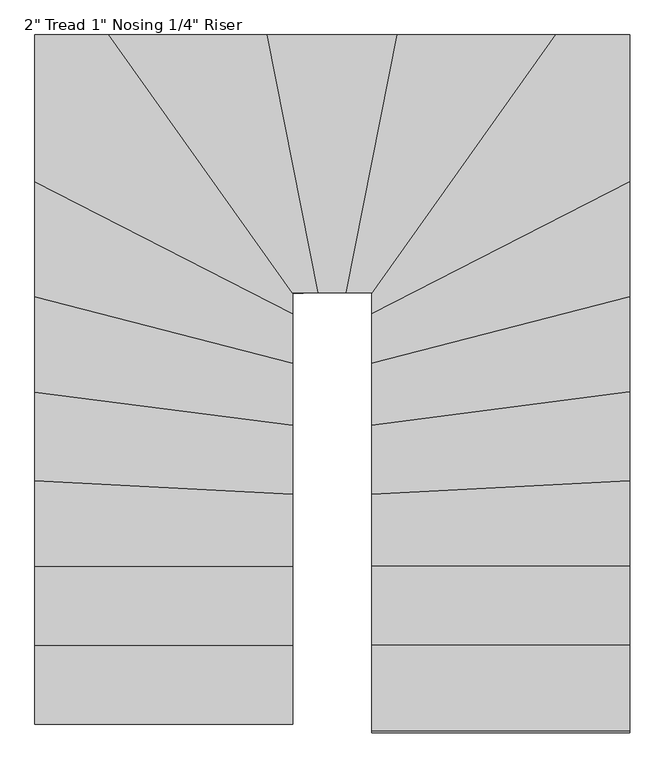
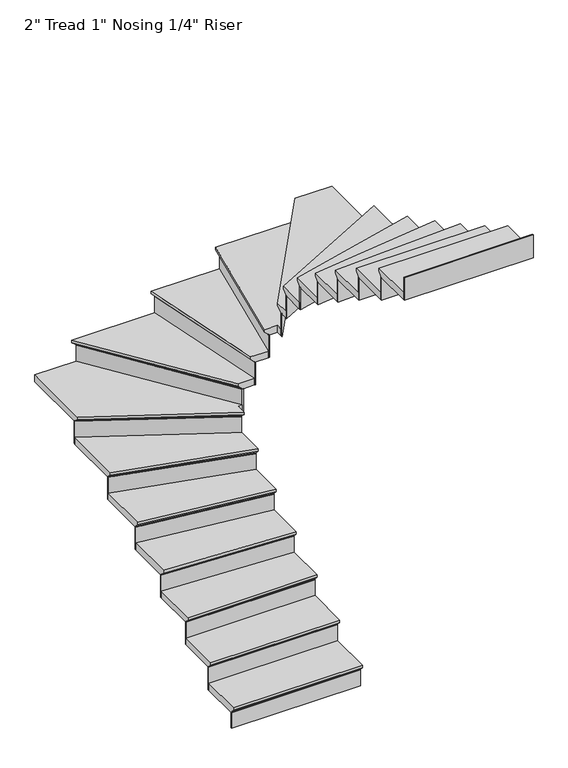
"""IFC4 building model written with IfcOpenShell, lengths in millimetres: stair flight geometry."""

from ifc_helpers import new_model, si_unit, origin, place, context, project, spatial, faceted_brep, source, transform, mapped, element, save


def stair_flight_4b86e887(model_context):
    return source(origin(), model_context, "Body", "Brep", [
        faceted_brep([(-715.0890964, 3647.9718401, 3350.6833333), (-715.0890964, 3647.9718401, 3369.7333333), (-1629.4890964, 3647.9718401, 3369.7333333), (-1629.4890964, 3647.9718401, 3350.6833333), (-715.0890964, 3673.3718401, 3325.2833333), (-1629.4890964, 3673.3718401, 3325.2833333), (-715.0890964, 3952.7718401, 3369.7333333), (-1629.4890964, 3952.7718401, 3369.7333333), (-1629.4890964, 3673.3718401, 3318.9333333), (-1629.4890964, 3952.7718401, 3318.9333333), (-715.0890964, 3952.7718401, 3318.9333333), (-715.0890964, 3673.3718401, 3318.9333333)], [[[0, 1, 2, 3]], [[4, 0, 3, 5]], [[2, 1, 6, 7]], [[8, 9, 10, 11]], [[2, 7, 9, 8, 5, 3]], [[8, 11, 4, 5]], [[6, 1, 0, 4, 11, 10]], [[7, 6, 10, 9]]]),
        faceted_brep([(-715.0890964, 3673.3718401, 3318.9333333), (-715.0890964, 3673.3718401, 3200.4), (-715.0890964, 3679.7218401, 3200.4), (-715.0890964, 3679.7218401, 3318.9333333), (-1629.4890964, 3673.3718401, 3318.9333333), (-1629.4890964, 3679.7218401, 3318.9333333), (-1629.4890964, 3679.7218401, 3200.4), (-1629.4890964, 3673.3718401, 3200.4)], [[[0, 1, 2, 3]], [[4, 5, 6, 7]], [[1, 0, 4, 7]], [[2, 1, 7, 6]], [[3, 2, 6, 5]], [[0, 3, 5, 4]]]),
        faceted_brep([(-715.0890964, 3952.7718401, 3488.2666667), (-715.0890964, 3952.7718401, 3318.9333333), (-715.0890964, 3959.1218401, 3318.9333333), (-715.0890964, 3959.1218401, 3488.2666667), (-1629.4890964, 3952.7718401, 3488.2666667), (-1629.4890964, 3959.1218401, 3488.2666667), (-1629.4890964, 3959.1218401, 3318.9333333), (-1629.4890964, 3952.7718401, 3318.9333333)], [[[0, 1, 2, 3]], [[4, 5, 6, 7]], [[1, 0, 4, 7]], [[2, 1, 7, 6]], [[3, 2, 6, 5]], [[0, 3, 5, 4]]]),
        faceted_brep([(-1629.4890964, 3927.3718401, 3539.0666667), (-715.0890964, 3927.3718401, 3539.0666667), (-715.0890964, 4232.1718401, 3539.0666667), (-1629.4890964, 4232.1718401, 3539.0666667), (-1629.4890964, 3952.7718401, 3488.2666667), (-1629.4890964, 4232.1718401, 3488.2666667), (-715.0890964, 4232.1718401, 3488.2666667), (-715.0890964, 3952.7718401, 3488.2666667), (-1629.4890964, 3952.7718401, 3494.6166667), (-1629.4890964, 3927.3718401, 3520.0166667), (-715.0890964, 3952.7718401, 3494.6166667), (-715.0890964, 3927.3718401, 3520.0166667)], [[[0, 1, 2, 3]], [[4, 5, 6, 7]], [[0, 3, 5, 4, 8, 9]], [[4, 7, 10, 8]], [[2, 1, 11, 10, 7, 6]], [[3, 2, 6, 5]], [[11, 1, 0, 9]], [[10, 11, 9, 8]]]),
        faceted_brep([(-715.0890964, 4232.1718401, 3657.6), (-715.0890964, 4232.1718401, 3488.2666667), (-715.0890964, 4238.5218401, 3488.2666667), (-715.0890964, 4238.5218401, 3657.6), (-1629.4890964, 4232.1718401, 3657.6), (-1629.4890964, 4238.5218401, 3657.6), (-1629.4890964, 4238.5218401, 3488.2666667), (-1629.4890964, 4232.1718401, 3488.2666667)], [[[0, 1, 2, 3]], [[4, 5, 6, 7]], [[1, 0, 4, 7]], [[2, 1, 7, 6]], [[3, 2, 6, 5]], [[0, 3, 5, 4]]]),
        faceted_brep([(-1629.4890964, 4206.7718401, 3708.4), (-715.0890964, 4206.7718401, 3708.4), (-715.0890964, 4487.8390016, 3708.4), (-1629.4890964, 4535.373272, 3708.4), (-1629.4890964, 4232.1718401, 3657.6), (-1629.4890964, 4535.373272, 3657.6), (-715.0890964, 4487.8390016, 3657.6), (-715.0890964, 4232.1718401, 3657.6), (-1629.4890964, 4232.1718401, 3663.95), (-1629.4890964, 4206.7718401, 3689.35), (-715.0890964, 4232.1718401, 3663.95), (-715.0890964, 4206.7718401, 3689.35)], [[[0, 1, 2, 3]], [[4, 5, 6, 7]], [[0, 3, 5, 4, 8, 9]], [[4, 7, 10, 8]], [[2, 1, 11, 10, 7, 6]], [[3, 2, 6, 5]], [[11, 1, 0, 9]], [[10, 11, 9, 8]]]),
        faceted_brep([(-715.0890964, 4487.8390016, 3826.9333333), (-715.0890964, 4487.8390016, 3657.6), (-715.0890964, 4494.1975757, 3657.6), (-715.0890964, 4494.1975757, 3826.9333333), (-1629.4890964, 4535.373272, 3826.9333333), (-1629.4890964, 4541.7318461, 3826.9333333), (-1629.4890964, 4541.7318461, 3657.6), (-1629.4890964, 4535.373272, 3657.6)], [[[0, 1, 2, 3]], [[4, 5, 6, 7]], [[1, 0, 4, 7]], [[2, 1, 7, 6]], [[3, 2, 6, 5]], [[0, 3, 5, 4]]]),
        faceted_brep([(-1629.4890964, 4509.9389753, 3877.7333333), (-715.0890964, 4462.4047049, 3877.7333333), (-715.0890964, 4732.0057014, 3877.7333333), (-1629.4890964, 4850.361753, 3877.7333333), (-1629.4890964, 4535.373272, 3826.9333333), (-1629.4890964, 4850.361753, 3826.9333333), (-715.0890964, 4732.0057014, 3826.9333333), (-715.0890964, 4487.8390016, 3826.9333333), (-1629.4890964, 4535.373272, 3833.2833333), (-1629.4890964, 4509.9389753, 3858.6833333), (-715.0890964, 4487.8390016, 3833.2833333), (-715.0890964, 4462.4047049, 3858.6833333)], [[[0, 1, 2, 3]], [[4, 5, 6, 7]], [[0, 3, 5, 4, 8, 9]], [[4, 7, 10, 8]], [[2, 1, 11, 10, 7, 6]], [[3, 2, 6, 5]], [[11, 1, 0, 9]], [[10, 11, 9, 8]]]),
        faceted_brep([(-715.0890964, 4732.0057014, 3996.2666667), (-715.0890964, 4732.0057014, 3826.9333333), (-715.0890964, 4738.4086732, 3826.9333333), (-715.0890964, 4738.4086732, 3996.2666667), (-1629.4890964, 4850.361753, 3996.2666667), (-1629.4890964, 4856.7647248, 3996.2666667), (-1629.4890964, 4856.7647248, 3826.9333333), (-1629.4890964, 4850.361753, 3826.9333333)], [[[0, 1, 2, 3]], [[4, 5, 6, 7]], [[1, 0, 4, 7]], [[2, 1, 7, 6]], [[3, 2, 6, 5]], [[0, 3, 5, 4]]]),
        faceted_brep([(-1629.4890964, 4824.7498659, 4047.0666667), (-715.0890964, 4706.3938143, 4047.0666667), (-715.0890964, 4953.6329239, 4047.0666667), (-1629.4890964, 5188.7633713, 4047.0666667), (-1629.4890964, 4850.361753, 3996.2666667), (-1629.4890964, 5188.7633713, 3996.2666667), (-715.0890964, 4953.6329239, 3996.2666667), (-715.0890964, 4732.0057014, 3996.2666667), (-1629.4890964, 4850.361753, 4002.6166667), (-1629.4890964, 4824.7498659, 4028.0166667), (-715.0890964, 4732.0057014, 4002.6166667), (-715.0890964, 4706.3938143, 4028.0166667)], [[[0, 1, 2, 3]], [[4, 5, 6, 7]], [[0, 3, 5, 4, 8, 9]], [[4, 7, 10, 8]], [[2, 1, 11, 10, 7, 6]], [[3, 2, 6, 5]], [[11, 1, 0, 9]], [[10, 11, 9, 8]]]),
        faceted_brep([(-715.0890964, 4953.6329239, 4165.6), (-715.0890964, 4953.6329239, 3996.2666667), (-715.0890964, 4960.1895007, 3996.2666667), (-715.0890964, 4960.1895007, 4165.6), (-1629.4890964, 5188.7633713, 4165.6), (-1629.4890964, 5195.3199481, 4165.6), (-1629.4890964, 5195.3199481, 3996.2666667), (-1629.4890964, 5188.7633713, 3996.2666667)], [[[0, 1, 2, 3]], [[4, 5, 6, 7]], [[1, 0, 4, 7]], [[2, 1, 7, 6]], [[3, 2, 6, 5]], [[0, 3, 5, 4]]]),
        faceted_brep([(-1629.4890964, 5162.5370638, 4216.4), (-715.0890964, 4927.4066164, 4216.4), (-715.0890964, 5129.9795599, 4216.4), (-1629.4890964, 5598.8041813, 4216.4), (-1629.4890964, 5188.7633713, 4165.6), (-1629.4890964, 5598.8041813, 4165.6), (-715.0890964, 5129.9795599, 4165.6), (-715.0890964, 4953.6329239, 4165.6), (-1629.4890964, 5188.7633713, 4171.95), (-1629.4890964, 5162.5370638, 4197.35), (-715.0890964, 4953.6329239, 4171.95), (-715.0890964, 4927.4066164, 4197.35)], [[[0, 1, 2, 3]], [[4, 5, 6, 7]], [[0, 3, 5, 4, 8, 9]], [[4, 7, 10, 8]], [[2, 1, 11, 10, 7, 6]], [[3, 2, 6, 5]], [[11, 1, 0, 9]], [[10, 11, 9, 8]]]),
        faceted_brep([(-715.0890964, 5129.9795599, 4334.9333333), (-715.0890964, 5129.9795599, 4165.6), (-715.0890964, 5137.1155431, 4165.6), (-715.0890964, 5137.1155431, 4334.9333333), (-1629.4890964, 5598.8041813, 4334.9333333), (-1629.4890964, 5605.9401644, 4334.9333333), (-1629.4890964, 5605.9401644, 4165.6), (-1629.4890964, 5598.8041813, 4165.6)], [[[0, 1, 2, 3]], [[4, 5, 6, 7]], [[1, 0, 4, 7]], [[2, 1, 7, 6]], [[3, 2, 6, 5]], [[0, 3, 5, 4]]]),
        faceted_brep([(-1335.8079627, 6090.103532, 4385.7333333), (-1629.4890964, 6090.103532, 4385.7333333), (-1629.4890964, 5570.2602487, 4385.7333333), (-715.0890964, 5101.4356274, 4385.7333333), (-715.0890964, 5175.703532, 4385.7333333), (-685.5340135, 5175.703532, 4385.7333333), (-1629.4890964, 6090.103532, 4334.9333333), (-1335.8079627, 6090.103532, 4334.9333333), (-685.5340135, 5175.703532, 4334.9333333), (-715.0890964, 5175.703532, 4334.9333333), (-715.0890964, 5129.9795599, 4334.9333333), (-1629.4890964, 5598.8041813, 4334.9333333), (-1629.4890964, 5598.8041813, 4341.2833333), (-1629.4890964, 5570.2602487, 4366.6833333), (-715.0890964, 5129.9795599, 4341.2833333), (-715.0890964, 5101.4356274, 4366.6833333)], [[[0, 1, 2, 3, 4, 5]], [[6, 7, 8, 9, 10, 11]], [[1, 0, 7, 6]], [[2, 1, 6, 11, 12, 13]], [[11, 10, 14, 12]], [[4, 3, 15, 14, 10, 9]], [[5, 4, 9, 8]], [[0, 5, 8, 7]], [[15, 3, 2, 13]], [[14, 15, 13, 12]]]),
        faceted_brep([(-685.5340135, 5175.703532, 4504.2666667), (-685.5340135, 5175.703532, 4334.9333333), (-677.7420387, 5175.703532, 4334.9333333), (-677.7420387, 5175.703532, 4504.2666667), (-1335.8079627, 6090.103532, 4504.2666667), (-1328.0159879, 6090.103532, 4504.2666667), (-1328.0159879, 6090.103532, 4334.9333333), (-1335.8079627, 6090.103532, 4334.9333333)], [[[0, 1, 2, 3]], [[4, 5, 6, 7]], [[1, 0, 4, 7]], [[2, 1, 7, 6]], [[3, 2, 6, 5]], [[0, 3, 5, 4]]]),
        faceted_brep([(-1366.9758618, 6090.103532, 4555.0666667), (-716.7019127, 5175.703532, 4555.0666667), (-599.0799265, 5175.703532, 4555.0666667), (-779.3207828, 6090.103532, 4555.0666667), (-1335.8079627, 6090.103532, 4504.2666667), (-779.3207828, 6090.103532, 4504.2666667), (-599.0799265, 5175.703532, 4504.2666667), (-685.5340135, 5175.703532, 4504.2666667), (-1335.8079627, 6090.103532, 4510.6166667), (-1366.9758618, 6090.103532, 4536.0166667), (-685.5340135, 5175.703532, 4510.6166667), (-716.7019127, 5175.703532, 4536.0166667)], [[[0, 1, 2, 3]], [[4, 5, 6, 7]], [[0, 3, 5, 4, 8, 9]], [[4, 7, 10, 8]], [[2, 1, 11, 10, 7, 6]], [[3, 2, 6, 5]], [[11, 1, 0, 9]], [[10, 11, 9, 8]]]),
        faceted_brep([(-599.0799265, 5175.703532, 4673.6), (-599.0799265, 5175.703532, 4504.2666667), (-592.607741, 5175.703532, 4504.2666667), (-592.607741, 5175.703532, 4673.6), (-779.3207828, 6090.103532, 4673.6), (-772.8485973, 6090.103532, 4673.6), (-772.8485973, 6090.103532, 4504.2666667), (-779.3207828, 6090.103532, 4504.2666667)], [[[0, 1, 2, 3]], [[4, 5, 6, 7]], [[1, 0, 4, 7]], [[2, 1, 7, 6]], [[3, 2, 6, 5]], [[0, 3, 5, 4]]]),
        faceted_brep([(-805.2095245, 6090.103532, 4724.4), (-624.9686682, 5175.703532, 4724.4), (-499.9207828, 5175.703532, 4724.4), (-319.6799265, 6090.103532, 4724.4), (-779.3207828, 6090.103532, 4673.6), (-319.6799265, 6090.103532, 4673.6), (-499.9207828, 5175.703532, 4673.6), (-599.0799265, 5175.703532, 4673.6), (-779.3207828, 6090.103532, 4679.95), (-805.2095245, 6090.103532, 4705.35), (-599.0799265, 5175.703532, 4679.95), (-624.9686682, 5175.703532, 4705.35)], [[[0, 1, 2, 3]], [[4, 5, 6, 7]], [[0, 3, 5, 4, 8, 9]], [[4, 7, 10, 8]], [[2, 1, 11, 10, 7, 6]], [[3, 2, 6, 5]], [[11, 1, 0, 9]], [[10, 11, 9, 8]]]),
        faceted_brep([(-499.9207828, 5175.703532, 4842.9333333), (-499.9207828, 5175.703532, 4673.6), (-493.4485973, 5175.703532, 4673.6), (-493.4485973, 5175.703532, 4842.9333333), (-319.6799265, 6090.103532, 4842.9333333), (-313.207741, 6090.103532, 4842.9333333), (-313.207741, 6090.103532, 4673.6), (-319.6799265, 6090.103532, 4673.6)], [[[0, 1, 2, 3]], [[4, 5, 6, 7]], [[1, 0, 4, 7]], [[2, 1, 7, 6]], [[3, 2, 6, 5]], [[0, 3, 5, 4]]]),
        faceted_brep([(-345.5686682, 6090.103532, 4893.7333333), (-525.8095245, 5175.703532, 4893.7333333), (-435.6890964, 5175.703532, 4893.7333333), (-435.6890964, 5129.6080574, 4893.7333333), (247.3655683, 6090.103532, 4893.7333333), (-319.6799265, 6090.103532, 4842.9333333), (247.3655683, 6090.103532, 4842.9333333), (-435.6890964, 5129.6080574, 4842.9333333), (-435.6890964, 5175.703532, 4842.9333333), (-499.9207828, 5175.703532, 4842.9333333), (-319.6799265, 6090.103532, 4849.2833333), (-345.5686682, 6090.103532, 4874.6833333), (-499.9207828, 5175.703532, 4849.2833333), (-525.8095245, 5175.703532, 4874.6833333)], [[[0, 1, 2, 3, 4]], [[5, 6, 7, 8, 9]], [[0, 4, 6, 5, 10, 11]], [[5, 9, 12, 10]], [[2, 1, 13, 12, 9, 8]], [[3, 2, 8, 7]], [[4, 3, 7, 6]], [[13, 1, 0, 11]], [[12, 13, 11, 10]]]),
        faceted_brep([(-435.6890964, 5129.6080574, 5012.2666667), (-435.6890964, 5129.6080574, 4842.9333333), (-435.6890964, 5118.6511649, 4842.9333333), (-435.6890964, 5118.6511649, 5012.2666667), (247.3655683, 6090.103532, 5012.2666667), (255.1575431, 6090.103532, 5012.2666667), (255.1575431, 6090.103532, 4842.9333333), (247.3655683, 6090.103532, 4842.9333333)], [[[0, 1, 2, 3]], [[4, 5, 6, 7]], [[1, 0, 4, 7]], [[2, 1, 7, 6]], [[3, 2, 6, 5]], [[0, 3, 5, 4]]]),
        faceted_brep([(478.7109036, 5541.7163162, 5063.0666667), (478.7109036, 6090.103532, 5063.0666667), (216.1976691, 6090.103532, 5063.0666667), (-435.6890964, 5173.4356274, 5063.0666667), (-435.6890964, 5072.8916949, 5063.0666667), (478.7109036, 6090.103532, 5012.2666667), (478.7109036, 5541.7163162, 5012.2666667), (-435.6890964, 5072.8916949, 5012.2666667), (-435.6890964, 5129.6080574, 5012.2666667), (247.3655683, 6090.103532, 5012.2666667), (247.3655683, 6090.103532, 5018.6166667), (216.1976691, 6090.103532, 5044.0166667), (-435.6890964, 5129.6080574, 5018.6166667), (-435.6890964, 5173.4356274, 5044.0166667)], [[[0, 1, 2, 3, 4]], [[5, 6, 7, 8, 9]], [[1, 0, 6, 5]], [[2, 1, 5, 9, 10, 11]], [[9, 8, 12, 10]], [[4, 3, 13, 12, 8, 7]], [[0, 4, 7, 6]], [[13, 3, 2, 11]], [[12, 13, 11, 10]]]),
        faceted_brep([(-435.6890964, 5072.8916949, 5181.6), (-435.6890964, 5072.8916949, 5012.2666667), (-435.6890964, 5065.7557117, 5012.2666667), (-435.6890964, 5065.7557117, 5181.6), (478.7109036, 5541.7163162, 5181.6), (478.7109036, 5534.5803331, 5181.6), (478.7109036, 5534.5803331, 5012.2666667), (478.7109036, 5541.7163162, 5012.2666667)], [[[0, 1, 2, 3]], [[4, 5, 6, 7]], [[1, 0, 4, 7]], [[2, 1, 7, 6]], [[3, 2, 6, 5]], [[0, 3, 5, 4]]]),
        faceted_brep([(478.7109036, 5570.2602487, 5232.4), (-435.6890964, 5101.4356274, 5232.4), (-435.6890964, 4901.1803089, 5232.4), (478.7109036, 5136.3107563, 5232.4), (478.7109036, 5541.7163162, 5181.6), (478.7109036, 5136.3107563, 5181.6), (-435.6890964, 4901.1803089, 5181.6), (-435.6890964, 5072.8916949, 5181.6), (478.7109036, 5541.7163162, 5187.95), (478.7109036, 5570.2602487, 5213.35), (-435.6890964, 5072.8916949, 5187.95), (-435.6890964, 5101.4356274, 5213.35)], [[[0, 1, 2, 3]], [[4, 5, 6, 7]], [[0, 3, 5, 4, 8, 9]], [[4, 7, 10, 8]], [[2, 1, 11, 10, 7, 6]], [[3, 2, 6, 5]], [[11, 1, 0, 9]], [[10, 11, 9, 8]]]),
        faceted_brep([(-435.6890964, 4901.1803089, 5350.9333333), (-435.6890964, 4901.1803089, 5181.6), (-435.6890964, 4894.6237321, 5181.6), (-435.6890964, 4894.6237321, 5350.9333333), (478.7109036, 5136.3107563, 5350.9333333), (478.7109036, 5129.7541795, 5350.9333333), (478.7109036, 5129.7541795, 5181.6), (478.7109036, 5136.3107563, 5181.6)], [[[0, 1, 2, 3]], [[4, 5, 6, 7]], [[1, 0, 4, 7]], [[2, 1, 7, 6]], [[3, 2, 6, 5]], [[0, 3, 5, 4]]]),
        faceted_brep([(478.7109036, 5162.5370638, 5401.7333333), (-435.6890964, 4927.4066164, 5401.7333333), (-435.6890964, 4680.7819272, 5401.7333333), (478.7109036, 4799.1379788, 5401.7333333), (478.7109036, 5136.3107563, 5350.9333333), (478.7109036, 4799.1379788, 5350.9333333), (-435.6890964, 4680.7819272, 5350.9333333), (-435.6890964, 4901.1803089, 5350.9333333), (478.7109036, 5136.3107563, 5357.2833333), (478.7109036, 5162.5370638, 5382.6833333), (-435.6890964, 4901.1803089, 5357.2833333), (-435.6890964, 4927.4066164, 5382.6833333)], [[[0, 1, 2, 3]], [[4, 5, 6, 7]], [[0, 3, 5, 4, 8, 9]], [[4, 7, 10, 8]], [[2, 1, 11, 10, 7, 6]], [[3, 2, 6, 5]], [[11, 1, 0, 9]], [[10, 11, 9, 8]]]),
        faceted_brep([(-435.6890964, 4680.7819272, 5520.2666667), (-435.6890964, 4680.7819272, 5350.9333333), (-435.6890964, 4674.3789554, 5350.9333333), (-435.6890964, 4674.3789554, 5520.2666667), (478.7109036, 4799.1379788, 5520.2666667), (478.7109036, 4792.735007, 5520.2666667), (478.7109036, 4792.735007, 5350.9333333), (478.7109036, 4799.1379788, 5350.9333333)], [[[0, 1, 2, 3]], [[4, 5, 6, 7]], [[1, 0, 4, 7]], [[2, 1, 7, 6]], [[3, 2, 6, 5]], [[0, 3, 5, 4]]]),
        faceted_brep([(478.7109036, 4824.7498659, 5571.0666667), (-435.6890964, 4706.3938143, 5571.0666667), (-435.6890964, 4436.9704082, 5571.0666667), (478.7109036, 4484.5046786, 5571.0666667), (478.7109036, 4799.1379788, 5520.2666667), (478.7109036, 4484.5046786, 5520.2666667), (-435.6890964, 4436.9704082, 5520.2666667), (-435.6890964, 4680.7819272, 5520.2666667), (478.7109036, 4799.1379788, 5526.6166667), (478.7109036, 4824.7498659, 5552.0166667), (-435.6890964, 4680.7819272, 5526.6166667), (-435.6890964, 4706.3938143, 5552.0166667)], [[[0, 1, 2, 3]], [[4, 5, 6, 7]], [[0, 3, 5, 4, 8, 9]], [[4, 7, 10, 8]], [[2, 1, 11, 10, 7, 6]], [[3, 2, 6, 5]], [[11, 1, 0, 9]], [[10, 11, 9, 8]]]),
        faceted_brep([(-435.6890964, 4436.9704082, 5689.6), (-435.6890964, 4436.9704082, 5520.2666667), (-435.6890964, 4430.6118341, 5520.2666667), (-435.6890964, 4430.6118341, 5689.6), (478.7109036, 4484.5046786, 5689.6), (478.7109036, 4478.1461045, 5689.6), (478.7109036, 4478.1461045, 5520.2666667), (478.7109036, 4484.5046786, 5520.2666667)], [[[0, 1, 2, 3]], [[4, 5, 6, 7]], [[1, 0, 4, 7]], [[2, 1, 7, 6]], [[3, 2, 6, 5]], [[0, 3, 5, 4]]]),
        faceted_brep([(478.7109036, 4509.9389753, 5740.4), (-435.6890964, 4462.4047049, 5740.4), (-435.6890964, 4181.3718401, 5740.4), (478.7109036, 4181.3718401, 5740.4), (478.7109036, 4484.5046786, 5689.6), (478.7109036, 4181.3718401, 5689.6), (-435.6890964, 4181.3718401, 5689.6), (-435.6890964, 4436.9704082, 5689.6), (478.7109036, 4484.5046786, 5695.95), (478.7109036, 4509.9389753, 5721.35), (-435.6890964, 4436.9704082, 5695.95), (-435.6890964, 4462.4047049, 5721.35)], [[[0, 1, 2, 3]], [[4, 5, 6, 7]], [[0, 3, 5, 4, 8, 9]], [[4, 7, 10, 8]], [[2, 1, 11, 10, 7, 6]], [[3, 2, 6, 5]], [[11, 1, 0, 9]], [[10, 11, 9, 8]]]),
        faceted_brep([(-435.6890964, 4181.3718401, 5858.9333333), (-435.6890964, 4181.3718401, 5689.6), (-435.6890964, 4175.0218401, 5689.6), (-435.6890964, 4175.0218401, 5858.9333333), (478.7109036, 4181.3718401, 5858.9333333), (478.7109036, 4175.0218401, 5858.9333333), (478.7109036, 4175.0218401, 5689.6), (478.7109036, 4181.3718401, 5689.6)], [[[0, 1, 2, 3]], [[4, 5, 6, 7]], [[1, 0, 4, 7]], [[2, 1, 7, 6]], [[3, 2, 6, 5]], [[0, 3, 5, 4]]]),
        faceted_brep([(478.7109036, 4206.7718401, 5909.7333333), (-435.6890964, 4206.7718401, 5909.7333333), (-435.6890964, 3901.9718401, 5909.7333333), (478.7109036, 3901.9718401, 5909.7333333), (478.7109036, 4181.3718401, 5858.9333333), (478.7109036, 3901.9718401, 5858.9333333), (-435.6890964, 3901.9718401, 5858.9333333), (-435.6890964, 4181.3718401, 5858.9333333), (478.7109036, 4181.3718401, 5865.2833333), (478.7109036, 4206.7718401, 5890.6833333), (-435.6890964, 4181.3718401, 5865.2833333), (-435.6890964, 4206.7718401, 5890.6833333)], [[[0, 1, 2, 3]], [[4, 5, 6, 7]], [[0, 3, 5, 4, 8, 9]], [[4, 7, 10, 8]], [[2, 1, 11, 10, 7, 6]], [[3, 2, 6, 5]], [[11, 1, 0, 9]], [[10, 11, 9, 8]]]),
        faceted_brep([(-435.6890964, 3901.9718401, 6028.2666667), (-435.6890964, 3901.9718401, 5858.9333333), (-435.6890964, 3895.6218401, 5858.9333333), (-435.6890964, 3895.6218401, 6028.2666667), (478.7109036, 3901.9718401, 6028.2666667), (478.7109036, 3895.6218401, 6028.2666667), (478.7109036, 3895.6218401, 5858.9333333), (478.7109036, 3901.9718401, 5858.9333333)], [[[0, 1, 2, 3]], [[4, 5, 6, 7]], [[1, 0, 4, 7]], [[2, 1, 7, 6]], [[3, 2, 6, 5]], [[0, 3, 5, 4]]]),
        faceted_brep([(-435.6890964, 3622.5718401, 6197.6), (-435.6890964, 3622.5718401, 6028.2666667), (-435.6890964, 3616.2218401, 6028.2666667), (-435.6890964, 3616.2218401, 6197.6), (478.7109036, 3622.5718401, 6197.6), (478.7109036, 3616.2218401, 6197.6), (478.7109036, 3616.2218401, 6028.2666667), (478.7109036, 3622.5718401, 6028.2666667)], [[[0, 1, 2, 3]], [[4, 5, 6, 7]], [[1, 0, 4, 7]], [[2, 1, 7, 6]], [[3, 2, 6, 5]], [[0, 3, 5, 4]]]),
        faceted_brep([(478.7109036, 3927.3718401, 6079.0666667), (-435.6890964, 3927.3718401, 6079.0666667), (-435.6890964, 3622.5718401, 6079.0666667), (478.7109036, 3622.5718401, 6079.0666667), (478.7109036, 3901.9718401, 6028.2666667), (478.7109036, 3622.5718401, 6028.2666667), (-435.6890964, 3622.5718401, 6028.2666667), (-435.6890964, 3901.9718401, 6028.2666667), (478.7109036, 3901.9718401, 6034.6166667), (478.7109036, 3927.3718401, 6060.0166667), (-435.6890964, 3901.9718401, 6034.6166667), (-435.6890964, 3927.3718401, 6060.0166667)], [[[0, 1, 2, 3]], [[4, 5, 6, 7]], [[0, 3, 5, 4, 8, 9]], [[4, 7, 10, 8]], [[2, 1, 11, 10, 7, 6]], [[3, 2, 6, 5]], [[11, 1, 0, 9]], [[10, 11, 9, 8]]]),
    ])


if __name__ == "__main__":
    model = new_model("IFC4")
    model_context = context("Model", 3, world=origin())
    ifc_project = project(units=[si_unit("LENGTHUNIT", "METRE", prefix="MILLI")], contexts=[model_context])
    site = spatial("IfcSite", under=ifc_project)
    building = spatial("IfcBuilding", under=site)
    placement = place(None, origin())
    stair_flight_shape = stair_flight_4b86e887(model_context)
    element("IfcStairFlight", 1, ObjectType="2\" Tread 1\" Nosing 1/4\" Riser", at=placement, inside=building, context=model_context, shape_type="MappedRepresentation", body=[
        mapped(stair_flight_shape, transform((0.0, 0.0, 0.0), x_axis=(1.0, 0.0, 0.0), y_axis=(0.0, 1.0, 0.0), z_axis=(0.0, 0.0, 1.0))),
    ])
    save(model, "model.ifc")
